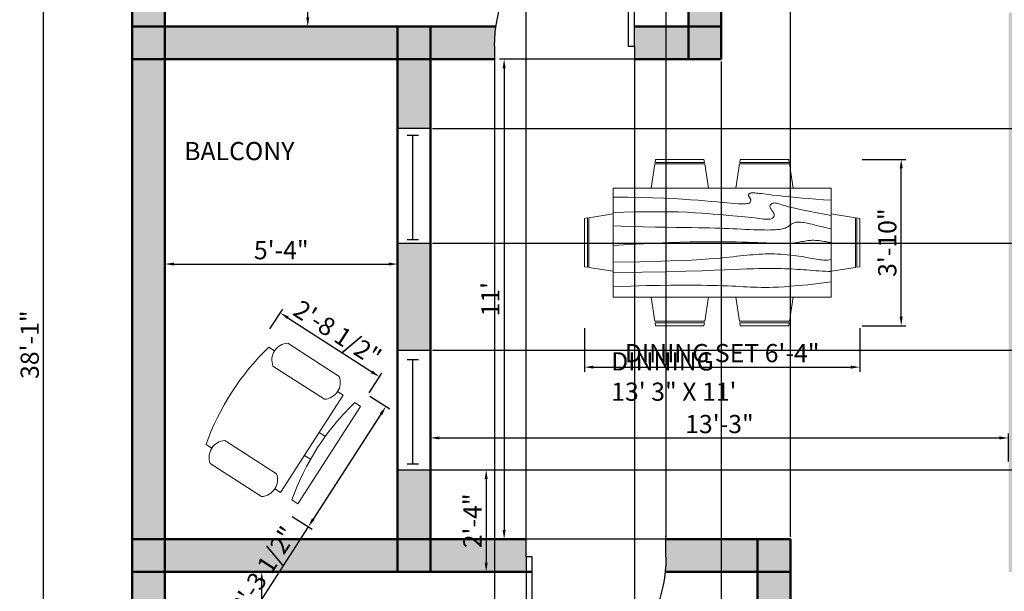
# Model space of a CAD drawing. Units: millimetres. Extents: x 3012 to 3478, y 929 to 1463.
# Tile 2 of 4: x 3012 to 3283, y 1118 to 1275. Entities that reach past the tile are written whole.
import ezdxf

# ---------------------------------------------------------------- set-up
doc = ezdxf.new("R2010")
doc.units = ezdxf.units.MM
for name, color, linetype, lineweight in [('A-ANNO-DIMS', 50, 'Continuous', 18), ('A-AREA-IDEN', 170, 'Continuous', 25), ('A-WALL-PATT', 252, 'Continuous', 13), ('doors', 130, 'Continuous', 25), ('furniture', 80, 'Continuous', 18), ('walls', 10, 'Continuous', 50), ('windows', 40, 'Continuous', 25)]:
    doc.layers.add(name, color=color, linetype=linetype, lineweight=lineweight)
doc.styles.get("Standard").update_dxf_attribs({"font": 'arial.ttf'})
doc.dimstyles.new('ISO-25', dxfattribs={"dimtxt": 5, "dimasz": 2.5, "dimexe": 1.25, "dimexo": 0.625, "dimtad": 1, "dimdec": 0, "dimlunit": 3, "dimtxsty": 'Standard', "dimcen": 2.5, "dimadec": 0, "dimazin": 0, "dimtfac": 1, "dimtdec": 0, "dimtmove": 0, "dimatfit": 3, "dimfxl": 1, "dimarcsym": 0})

# ---------------------------------------------------------------- blocks, each defined once
blk = doc.blocks.new('*U2')
for p, q in [((0, 0), (0, -6)), ((40, 0), (40, -6))]:
    blk.add_line(p, q)
blk.add_lwpolyline([(0, 0), (0, 40), (1.75, 40), (1.75, 0)], close=True)
blk.add_arc((0, 0), 40, 0, 90)
blk = doc.blocks.new('*U4')
for p, q in [((0, 4), (0, 0)), ((36, 4), (36, 0)), ((0, 2), (36, 2))]:
    blk.add_line(p, q)
blk = doc.blocks.new('Dining Set - 36 x 72 in.')
for p, q in [((-22, 27.5), (-22.1562, 26.50042)), ((-5.8416, 26.5), (-22.1534, 26.5)), ((-22, 27.5), (-6, 27.5)), ((-5.8437, 26.49966), (-6, 27.5)), ((6, 27.5), (5.8438, 26.50042)), ((22.1584, 26.5), (5.8466, 26.5)), ((6, 27.5), (22, 27.5)), ((22.1563, 26.49966), (22, 27.5)), ((-22.2343, 26.00059), (-23.4847, 17.99762)), ((-22.2304, 26), (-5.7608, 26)), ((-4.5152, 17.99762), (-5.7655, 25.99926)), ((5.7657, 26.00059), (4.5153, 17.99762)), ((5.7696, 26), (22.2392, 26)), ((23.4848, 17.99762), (22.2345, 25.99926)), ((36, 18), (-36, 18)), ((-36, 18), (-36, -18)), ((36, -18), (36, 18)), ((-45.5, 8), (-44.5004, 8.15617)), ((-45.5, 8), (-45.5, -8)), ((-44.5, -8.15843), (-44.5, 8.15338)), ((-44.0006, 8.23428), (-35.9976, 9.48474)), ((-44, 8.23041), (-44, -8.23915)), ((44.0006, 8.23428), (35.9976, 9.48474)), ((44, 8.23041), (44, -8.23915)), ((44.5, -8.15843), (44.5, 8.15338)), ((45.5, 8), (44.5005, 8.15617)), ((45.5, 8), (45.5, -8)), ((-44.4997, -8.15631), (-45.5, -8)), ((-35.9976, -9.48476), (-43.9993, -8.2345)), ((35.9976, -9.48476), (43.9993, -8.2345)), ((44.4997, -8.15631), (45.5, -8)), ((-36, -18), (36, -18)), ((-22.2343, -26.0006), (-23.4847, -17.99762)), ((-4.5152, -17.99762), (-5.7655, -25.99928)), ((5.7657, -26.0006), (4.5153, -17.99762)), ((23.4848, -17.99762), (22.2345, -25.99928)), ((-22.2304, -26), (-5.7608, -26)), ((5.7696, -26), (22.2392, -26)), ((-22, -27.5), (-22.1562, -26.50044)), ((-5.8416, -26.5), (-22.1534, -26.5)), ((-22, -27.5), (-6, -27.5)), ((-5.8437, -26.49967), (-6, -27.5)), ((6, -27.5), (5.8438, -26.50044)), ((22.1584, -26.5), (5.8466, -26.5)), ((6, -27.5), (22, -27.5)), ((22.1563, -26.49967), (22, -27.5))]:
    blk.add_line(p, q)
for points in [[(-36, 15), (-31.1772, 14.97754), (-26.8079, 14.91406), (-22.8538, 14.81543), (-19.276, 14.6875), (-16.0362, 14.53613), (-13.0957, 14.36718), (-10.4159, 14.18652), (-7.9583, 14), (-5.6904, 13.81315), (-3.6035, 13.63021), (-1.6954, 13.45508), (0.0365, 13.29166), (1.5945, 13.14388), (2.9811, 13.01562), (4.1988, 12.9108), (5.25, 12.83333), (6.1393, 12.78613), (6.8802, 12.76823), (7.4883, 12.77767), (7.9792, 12.8125), (8.3685, 12.87077), (8.6719, 12.95052), (8.9049, 13.0498), (9.0833, 13.16666), (9.2205, 13.29899), (9.3216, 13.44401), (9.3895, 13.59879), (9.4271, 13.76041), (9.4373, 13.92594), (9.4232, 14.09245), (9.3875, 14.257), (9.3333, 14.41666), (9.2638, 14.56917), (9.1836, 14.71484), (9.0975, 14.85465), (9.0104, 14.98958), (8.9272, 15.1206), (8.8529, 15.2487), (8.7922, 15.37483), (8.75, 15.5), (8.7305, 15.62467), (8.7344, 15.74739), (8.7617, 15.86621), (8.8125, 15.97916), (8.8867, 16.08431), (8.9844, 16.17968), (9.1055, 16.26334), (9.25, 16.33333), (9.4189, 16.38802), (9.6172, 16.42708), (9.8506, 16.45052), (10.125, 16.45833), (10.4463, 16.45052), (10.8203, 16.42708), (11.2529, 16.38802), (11.75, 16.33333), (12.3184, 16.26318), (12.9694, 16.17838), (13.7151, 16.07991), (14.5677, 15.96875), (15.5395, 15.84586), (16.6426, 15.71224), (17.8893, 15.56884), (19.2917, 15.41666), (20.859, 15.25667), (22.5879, 15.08984), (24.4721, 14.91715), (26.5052, 14.73958), (28.6809, 14.5581), (30.9929, 14.3737), (33.4347, 14.18733), (36, 14)], [(-36, 10), (-28.9766, 10.14274), (-23.1725, 10.20442), (-18.4241, 10.19775), (-14.5677, 10.13541), (-11.4399, 10.03011), (-8.877, 9.89453), (-6.7154, 9.74137), (-4.7917, 9.58333), (-2.9698, 9.43082), (-1.2246, 9.28515), (0.4415, 9.14534), (2.026, 9.01041), (3.5266, 8.87939), (4.9408, 8.7513), (6.266, 8.62516), (7.5, 8.5), (8.6411, 8.37549), (9.6914, 8.2539), (10.6538, 8.13818), (11.5312, 8.03125), (12.3267, 7.93603), (13.043, 7.85547), (13.6831, 7.79248), (14.25, 7.75), (14.7471, 7.7303), (15.1797, 7.73307), (15.5537, 7.75732), (15.875, 7.80208), (16.1494, 7.86637), (16.3828, 7.94922), (16.5811, 8.04964), (16.75, 8.16666), (16.8944, 8.29915), (17.0143, 8.44531), (17.1089, 8.60319), (17.1771, 8.77083), (17.218, 8.94629), (17.2305, 9.1276), (17.2137, 9.31282), (17.1667, 9.5), (17.0895, 9.6875), (16.987, 9.875), (16.8649, 10.0625), (16.7292, 10.25), (16.5856, 10.4375), (16.4401, 10.625), (16.2985, 10.8125), (16.1667, 11), (16.05, 11.18733), (15.9518, 11.3737), (15.8752, 11.5581), (15.8229, 11.73958), (15.798, 11.91715), (15.8034, 12.08984), (15.842, 12.25667), (15.9167, 12.41666), (16.0295, 12.56836), (16.1784, 12.70833), (16.3605, 12.83268), (16.5729, 12.9375), (16.8127, 13.01888), (17.0768, 13.07291), (17.3625, 13.0957), (17.6667, 13.08333), (17.9894, 13.03312), (18.3418, 12.94726), (18.7382, 12.82918), (19.1927, 12.68229), (19.7195, 12.51001), (20.3327, 12.31575), (21.0465, 12.10294), (21.875, 11.875), (22.8357, 11.63354), (23.959, 11.37304), (25.2786, 11.08618), (26.8282, 10.76562), (28.6414, 10.40405), (30.752, 9.99414), (33.1936, 9.52856), (36, 9)], [(-36, 5.5), (-30.7157, 5.3348), (-26.069, 5.20963), (-21.9946, 5.11767), (-18.4271, 5.05208), (-15.3009, 5.00602), (-12.5508, 4.97265), (-10.1112, 4.94515), (-7.9167, 4.91666), (-5.909, 4.88167), (-4.0586, 4.83984), (-2.3429, 4.79215), (-0.7396, 4.73958), (0.7739, 4.6831), (2.22, 4.6237), (3.6213, 4.56233), (5, 4.5), (6.373, 4.43782), (7.7344, 4.3776), (9.0723, 4.32129), (10.375, 4.27083), (11.6309, 4.22819), (12.8281, 4.19531), (13.9551, 4.17415), (15, 4.16666), (15.954, 4.17448), (16.819, 4.19791), (17.6001, 4.23698), (18.3021, 4.29166), (18.9299, 4.36198), (19.4883, 4.44791), (19.9823, 4.54948), (20.4167, 4.66666), (20.7969, 4.79899), (21.1302, 4.94401), (21.4245, 5.09879), (21.6875, 5.26041), (21.9271, 5.42594), (22.1511, 5.59245), (22.3672, 5.757), (22.5834, 5.91666), (22.8065, 6.06868), (23.0404, 6.21093), (23.2879, 6.34147), (23.5521, 6.45833), (23.8358, 6.55957), (24.142, 6.64323), (24.4735, 6.70735), (24.8334, 6.75), (25.2235, 6.76969), (25.642, 6.76692), (26.0858, 6.74267), (26.5521, 6.69791), (27.0379, 6.63362), (27.5404, 6.55078), (28.0565, 6.45036), (28.5834, 6.33333), (29.1242, 6.19987), (29.7071, 6.04687), (30.3661, 5.87044), (31.1354, 5.66666), (32.0493, 5.43164), (33.142, 5.16146), (34.4475, 4.85221), (36, 4.5)], [(-36, -1), (-30.7915, -0.6591), (-26.0195, -0.38216), (-21.6519, -0.16284), (-17.6563, 0.00521), (-14.0005, 0.12833), (-10.6523, 0.21289), (-7.5796, 0.26522), (-4.75, 0.29166), (-2.134, 0.29793), (0.2878, 0.28711), (2.5317, 0.26163), (4.6146, 0.22396), (6.5529, 0.17651), (8.3633, 0.12174), (10.0623, 0.06209), (11.6667, 0), (13.1899, -0.06201), (14.6341, -0.1211), (15.9982, -0.17432), (17.2813, -0.21875), (18.4823, -0.25147), (19.6003, -0.26953), (20.6343, -0.27002), (21.5834, -0.25), (22.4481, -0.20768), (23.2357, -0.14584), (23.9549, -0.06836), (24.6146, 0.02083), (25.2235, 0.11784), (25.7904, 0.21875), (26.3241, 0.31966), (26.8334, 0.41666), (27.3265, 0.50618), (27.8099, 0.58593), (28.2894, 0.65397), (28.7709, 0.70833), (29.2601, 0.74707), (29.763, 0.76823), (30.2855, 0.76985), (30.8334, 0.75), (31.4088, 0.70784), (31.9994, 0.64713), (32.589, 0.57275), (33.1615, 0.48958), (33.7008, 0.4025), (34.1908, 0.3164), (34.6153, 0.23616), (34.9584, 0.16666), (35.2099, 0.11165), (35.3848, 0.07031), (35.504, 0.04069), (35.5886, 0.02083), (35.6594, 0.00879), (35.7377, 0.0026), (35.8442, 0.00032), (36, 0)], [(-36, -6.5), (-27.1843, -6.31267), (-20.084, -6.1263), (-14.469, -5.9419), (-10.1094, -5.76042), (-6.7752, -5.58285), (-4.2363, -5.41016), (-2.2629, -5.24333), (-0.625, -5.08334), (0.8708, -4.93099), (2.2715, -4.78646), (3.5872, -4.64974), (4.8281, -4.52084), (6.0046, -4.39974), (7.127, -4.28646), (8.2053, -4.18099), (9.25, -4.08334), (10.2705, -3.99382), (11.2734, -3.91407), (12.2647, -3.84603), (13.25, -3.79167), (14.2354, -3.75293), (15.2266, -3.73177), (16.2295, -3.73015), (17.25, -3.75), (18.2912, -3.79248), (19.3451, -3.85547), (20.4009, -3.93604), (21.4479, -4.03125), (22.4754, -4.13819), (23.4727, -4.25391), (24.4289, -4.37549), (25.3334, -4.5), (26.1785, -4.62492), (26.9694, -4.74935), (27.7145, -4.87281), (28.4219, -4.99479), (29.1, -5.11483), (29.7572, -5.23242), (30.4016, -5.34709), (31.0417, -5.45834), (31.6837, -5.56437), (32.3262, -5.65821), (32.9658, -5.73153), (33.599, -5.77604), (34.2224, -5.78345), (34.8327, -5.74545), (35.4264, -5.65373), (36, -5.5)], [(-36, -10), (-26.4022, -9.81299), (-18.4675, -9.62891), (-11.9839, -9.45069), (-6.7396, -9.28125), (-2.5226, -9.12354), (0.8789, -8.98047), (3.6769, -8.85498), (6.0833, -8.75), (8.2767, -8.66765), (10.3021, -8.60677), (12.1712, -8.56543), (13.8958, -8.54167), (15.4876, -8.53353), (16.9583, -8.53907), (18.3197, -8.55632), (19.5834, -8.58334), (20.7616, -8.61841), (21.8685, -8.66081), (22.9188, -8.71004), (23.9271, -8.76563), (24.9081, -8.82707), (25.8763, -8.89388), (26.8465, -8.96558), (27.8334, -9.04167), (28.8474, -9.12118), (29.8828, -9.20117), (30.93, -9.27824), (31.9792, -9.34896), (33.0205, -9.40991), (34.0443, -9.45768), (35.0407, -9.48885), (36, -9.5)], [(-36, -14.5), (-30.0881, -14.33513), (-25.0332, -14.21224), (-20.7312, -14.12647), (-17.0781, -14.07292), (-13.97, -14.04671), (-11.3027, -14.04297), (-8.9724, -14.05681), (-6.875, -14.08334), (-4.9224, -14.11833), (-3.0905, -14.16016), (-1.3709, -14.20785), (0.2448, -14.26042), (1.7647, -14.3169), (3.1973, -14.3763), (4.5507, -14.43767), (5.8333, -14.5), (7.0554, -14.5621), (8.235, -14.62175), (9.3922, -14.67652), (10.5469, -14.72396), (11.7192, -14.76164), (12.929, -14.78711), (14.1965, -14.79794), (15.5417, -14.79167), (16.9933, -14.76424), (18.6152, -14.70508), (20.4804, -14.60197), (22.6615, -14.44271), (25.2312, -14.21509), (28.2624, -13.9069), (31.8277, -13.50594), (36, -13)]]:
    blk.add_lwpolyline(points)
blk = doc.blocks.new('Chair - Desk')
for p, q in [((-8.5, 0), (-8.5, -1)), ((-8.5, 0), (8.5, 0)), ((8.5, 0), (8.5, -1)), ((-2, -3), (-2, -1.9355)), ((2, -1.9576), (2, -3)), ((-8.5, -3), (-8.5, -4)), ((-8.5, -3), (8.5, -3)), ((8.5, -3), (8.5, -4)), ((-10.5, -5), (-10.5, -14)), ((-6.5, -14), (-6.5, -5)), ((6.5, -5), (6.5, -14)), ((10.5, -14), (10.5, -5)), ((-8.5, -15), (-8.5, -16)), ((8.5, -15), (8.5, -16))]:
    blk.add_line(p, q)
for centre, radius, start, end in [((0, 34.625), 36.625, 256.5803, 283.4197), ((-8.5, -6.5), 2.5, 36.8699, 143.1301), ((8.5, -6.5), 2.5, 36.8699, 143.1301), ((-8.5, -12.5), 2.5, 216.8699, 323.1301), ((8.5, -12.5), 2.5, 216.8699, 323.1301), ((0, 19.625), 36.625, 256.5803, 283.4197)]:
    blk.add_arc(centre, radius, start, end)
blk = doc.blocks.new('*D13')
at = {"layer": 'A-ANNO-DIMS', "color": 0, "lineweight": -2, "transparency": 16777216}
for p, q in [((3089.79, 1405.44), (3092.75, 1405.44)), ((3091.5, 1275.94), (3091.5, 1402.94)), ((3089.79, 1273.44), (3092.75, 1273.44))]:
    blk.add_line(p, q, dxfattribs=at)
at = {"layer": 'A-ANNO-DIMS', "color": 0, "transparency": 16777216}
for points in [[(3091.08, 1402.94), (3091.91, 1402.94), (3091.5, 1405.44)], [(3091.08, 1275.94), (3091.91, 1275.94), (3091.5, 1273.44)]]:
    blk.add_solid(points, dxfattribs=at)
at = {"layer": 'Defpoints', "color": 0, "transparency": 16777216}
for p in [(3089.17, 1405.44), (3091.5, 1405.44), (3089.17, 1273.44)]:
    blk.add_point(p, dxfattribs=at)
at = {"layer": 'A-ANNO-DIMS', "color": 0, "transparency": 16777216, "insert": (3088.36, 1339.44), "char_height": 5, "attachment_point": 5, "rotation": 90}
blk.add_mtext("11'", dxfattribs=at)
blk = doc.blocks.new('*D17')
at = {"layer": 'A-ANNO-DIMS', "color": 0, "lineweight": -2, "transparency": 16777216}
for p, q in [((3052.21, 1203.36), (3052.21, 1209.37)), ((3054.71, 1208.12), (3113.71, 1208.12)), ((3116.21, 1203.36), (3116.21, 1209.37))]:
    blk.add_line(p, q, dxfattribs=at)
at = {"layer": 'A-ANNO-DIMS', "color": 0, "transparency": 16777216}
for points in [[(3054.71, 1208.53), (3054.71, 1207.7), (3052.21, 1208.12)], [(3113.71, 1208.53), (3113.71, 1207.7), (3116.21, 1208.12)]]:
    blk.add_solid(points, dxfattribs=at)
at = {"layer": 'Defpoints', "color": 0, "transparency": 16777216}
for p in [(3116.21, 1208.12), (3052.21, 1202.73), (3116.21, 1202.73)]:
    blk.add_point(p, dxfattribs=at)
at = {"layer": 'A-ANNO-DIMS', "color": 0, "transparency": 16777216, "insert": (3084.21, 1211.28), "char_height": 5, "attachment_point": 5}
blk.add_mtext('5\'-4"', dxfattribs=at)
blk = doc.blocks.new('*D19')
at = {"layer": 'A-ANNO-DIMS', "color": 0, "lineweight": -2, "transparency": 16777216}
for p, q in [((3065.42, 1123.44), (3080.09, 1123.44)), ((3078.84, 968.94), (3078.84, 1120.94)), ((3065.42, 966.44), (3080.09, 966.44))]:
    blk.add_line(p, q, dxfattribs=at)
at = {"layer": 'A-ANNO-DIMS', "color": 0, "transparency": 16777216}
for points in [[(3078.43, 1120.94), (3079.26, 1120.94), (3078.84, 1123.44)], [(3078.43, 968.94), (3079.26, 968.94), (3078.84, 966.44)]]:
    blk.add_solid(points, dxfattribs=at)
at = {"layer": 'Defpoints', "color": 0, "transparency": 16777216}
for p in [(3064.8, 1123.44), (3078.84, 1123.44), (3064.8, 966.44)]:
    blk.add_point(p, dxfattribs=at)
at = {"layer": 'A-ANNO-DIMS', "color": 0, "transparency": 16777216, "insert": (3075.66, 1044.94), "char_height": 5, "attachment_point": 5, "rotation": 90}
blk.add_mtext('13\'-1"', dxfattribs=at)
blk = doc.blocks.new('*D25')
at = {"layer": 'A-ANNO-DIMS', "color": 0, "lineweight": -2, "transparency": 16777216}
for p, q in [((3125.21, 1153.8), (3125.21, 1161.53)), ((3127.71, 1160.28), (3281.71, 1160.28)), ((3284.21, 1153.8), (3284.21, 1161.53))]:
    blk.add_line(p, q, dxfattribs=at)
at = {"layer": 'A-ANNO-DIMS', "color": 0, "transparency": 16777216}
for points in [[(3127.71, 1160.7), (3127.71, 1159.86), (3125.21, 1160.28)], [(3281.71, 1160.7), (3281.71, 1159.86), (3284.21, 1160.28)]]:
    blk.add_solid(points, dxfattribs=at)
at = {"layer": 'Defpoints', "color": 0, "transparency": 16777216}
for p in [(3284.21, 1160.28), (3125.21, 1153.17), (3284.21, 1153.17)]:
    blk.add_point(p, dxfattribs=at)
at = {"layer": 'A-ANNO-DIMS', "color": 0, "transparency": 16777216, "insert": (3204.71, 1163.46), "char_height": 5, "attachment_point": 5}
blk.add_mtext('13\'-3"', dxfattribs=at)
blk = doc.blocks.new('*D26')
at = {"layer": 'A-ANNO-DIMS', "color": 0, "lineweight": -2, "transparency": 16777216}
for p, q in [((3195.59, 1264.44), (3144.25, 1264.44)), ((3145.5, 1261.94), (3145.5, 1134.94)), ((3195.59, 1132.44), (3144.25, 1132.44))]:
    blk.add_line(p, q, dxfattribs=at)
at = {"layer": 'A-ANNO-DIMS', "color": 0, "transparency": 16777216}
for points in [[(3145.08, 1261.94), (3145.92, 1261.94), (3145.5, 1264.44)], [(3145.08, 1134.94), (3145.92, 1134.94), (3145.5, 1132.44)]]:
    blk.add_solid(points, dxfattribs=at)
at = {"layer": 'Defpoints', "color": 0, "transparency": 16777216}
for p in [(3196.21, 1264.44), (3145.5, 1132.44), (3196.21, 1132.44)]:
    blk.add_point(p, dxfattribs=at)
at = {"layer": 'A-ANNO-DIMS', "color": 0, "transparency": 16777216, "insert": (3142.36, 1198.44), "char_height": 5, "attachment_point": 5, "rotation": 90}
blk.add_mtext("11'", dxfattribs=at)
blk = doc.blocks.new('*D34')
at = {"layer": 'A-ANNO-DIMS', "color": 0, "lineweight": -2, "transparency": 16777216}
for p, q in [((3167.57, 1190.5), (3167.57, 1178.51)), ((3243.33, 1190.5), (3243.33, 1178.51)), ((3170.07, 1179.76), (3240.83, 1179.76))]:
    blk.add_line(p, q, dxfattribs=at)
at = {"layer": 'A-ANNO-DIMS', "color": 0, "transparency": 16777216}
for points in [[(3170.07, 1180.17), (3170.07, 1179.34), (3167.57, 1179.76)], [(3240.83, 1180.17), (3240.83, 1179.34), (3243.33, 1179.76)]]:
    blk.add_solid(points, dxfattribs=at)
at = {"layer": 'Defpoints', "color": 0, "transparency": 16777216}
for p in [(3167.57, 1191.12), (3243.33, 1191.12), (3243.33, 1179.76)]:
    blk.add_point(p, dxfattribs=at)
at = {"layer": 'A-ANNO-DIMS', "color": 0, "transparency": 16777216, "insert": (3205.45, 1182.97), "char_height": 5, "attachment_point": 5}
blk.add_mtext('DINING SET 6\'-4"', dxfattribs=at)
blk = doc.blocks.new('*D35')
at = {"layer": 'A-ANNO-DIMS', "color": 0, "lineweight": -2, "transparency": 16777216}
for p, q in [((3243.95, 1236.91), (3255.94, 1236.91)), ((3254.69, 1193.62), (3254.69, 1234.41)), ((3243.95, 1191.12), (3255.94, 1191.12))]:
    blk.add_line(p, q, dxfattribs=at)
at = {"layer": 'A-ANNO-DIMS', "color": 0, "transparency": 16777216}
for points in [[(3254.27, 1234.41), (3255.11, 1234.41), (3254.69, 1236.91)], [(3254.27, 1193.62), (3255.11, 1193.62), (3254.69, 1191.12)]]:
    blk.add_solid(points, dxfattribs=at)
at = {"layer": 'Defpoints', "color": 0, "transparency": 16777216}
for p in [(3243.33, 1236.91), (3254.69, 1236.91), (3243.33, 1191.12)]:
    blk.add_point(p, dxfattribs=at)
at = {"layer": 'A-ANNO-DIMS', "color": 0, "transparency": 16777216, "insert": (3251.51, 1214.01), "char_height": 5, "attachment_point": 5, "rotation": 90}
blk.add_mtext('3\'-10"', dxfattribs=at)
blk = doc.blocks.new('*D40')
at = {"layer": 'A-ANNO-DIMS', "color": 0, "lineweight": -2, "transparency": 16777216}
for p, q in [((3108.55, 1171.79), (3114.04, 1168.25)), ((3111.63, 1166.83), (3093, 1137.95)), ((3087.21, 1138.72), (3092.7, 1135.18)), ((3091.65, 1135.85), (3063.29, 1091.9))]:
    blk.add_line(p, q, dxfattribs=at)
at = {"layer": 'A-ANNO-DIMS', "color": 0, "transparency": 16777216}
for points in [[(3111.28, 1167.05), (3111.98, 1166.6), (3112.99, 1168.93)], [(3092.65, 1138.18), (3093.35, 1137.73), (3091.65, 1135.85)]]:
    blk.add_solid(points, dxfattribs=at)
at = {"layer": 'Defpoints', "color": 0, "transparency": 16777216}
for p in [(3108.03, 1172.13), (3086.69, 1139.06), (3091.65, 1135.85)]:
    blk.add_point(p, dxfattribs=at)
at = {"layer": 'A-ANNO-DIMS', "color": 0, "transparency": 16777216, "insert": (3074.09, 1114.57), "char_height": 5, "attachment_point": 5, "rotation": 57.1659}
blk.add_mtext('CHAIR 3\'-3 1/2"', dxfattribs=at)
blk = doc.blocks.new('*D41')
at = {"layer": 'A-ANNO-DIMS', "color": 0, "lineweight": -2, "transparency": 16777216}
for p, q in [((3081.07, 1190.27), (3084.61, 1195.75)), ((3086.03, 1193.35), (3109.13, 1178.44)), ((3108.37, 1172.65), (3111.91, 1178.14))]:
    blk.add_line(p, q, dxfattribs=at)
at = {"layer": 'A-ANNO-DIMS', "color": 0, "transparency": 16777216}
for points in [[(3086.26, 1193.7), (3085.81, 1193), (3083.93, 1194.7)], [(3109.35, 1178.79), (3108.9, 1178.09), (3111.23, 1177.09)]]:
    blk.add_solid(points, dxfattribs=at)
at = {"layer": 'Defpoints', "color": 0, "transparency": 16777216}
for p in [(3080.73, 1189.74), (3111.23, 1177.09), (3108.03, 1172.13)]:
    blk.add_point(p, dxfattribs=at)
at = {"layer": 'A-ANNO-DIMS', "color": 0, "transparency": 16777216, "insert": (3099.32, 1188.59), "char_height": 5, "attachment_point": 5, "rotation": 327.1659}
blk.add_mtext('2\'-8 1/2"', dxfattribs=at)
blk = doc.blocks.new('*D42')
at = {"layer": 'A-ANNO-DIMS', "color": 0, "lineweight": -2, "transparency": 16777216}
for p, q in [((3042.59, 1414.44), (3017.61, 1414.44)), ((3018.86, 959.94), (3018.86, 1411.94)), ((3042.59, 957.44), (3017.61, 957.44))]:
    blk.add_line(p, q, dxfattribs=at)
at = {"layer": 'A-ANNO-DIMS', "color": 0, "transparency": 16777216}
for points in [[(3018.45, 1411.94), (3019.28, 1411.94), (3018.86, 1414.44)], [(3018.45, 959.94), (3019.28, 959.94), (3018.86, 957.44)]]:
    blk.add_solid(points, dxfattribs=at)
at = {"layer": 'Defpoints', "color": 0, "transparency": 16777216}
for p in [(3018.86, 1414.44), (3043.21, 1414.44), (3043.21, 957.44)]:
    blk.add_point(p, dxfattribs=at)
at = {"layer": 'A-ANNO-DIMS', "color": 0, "transparency": 16777216, "insert": (3015.68, 1185.94), "char_height": 5, "attachment_point": 5, "rotation": 90}
blk.add_mtext('38\'-1"', dxfattribs=at)
blk = doc.blocks.new('*D57')
at = {"layer": 'A-ANNO-DIMS', "color": 0, "lineweight": -2, "transparency": 16777216}
for p, q in [((3142.87, 1263.82), (3142.87, 931.84)), ((3181.32, 1263.82), (3181.32, 931.84)), ((3145.37, 933.09), (3178.82, 933.09))]:
    blk.add_line(p, q, dxfattribs=at)
at = {"layer": 'A-ANNO-DIMS', "color": 0, "transparency": 16777216}
for points in [[(3145.37, 933.51), (3145.37, 932.68), (3142.87, 933.09)], [(3178.82, 933.51), (3178.82, 932.68), (3181.32, 933.09)]]:
    blk.add_solid(points, dxfattribs=at)
at = {"layer": 'Defpoints', "color": 0, "transparency": 16777216}
for p in [(3142.87, 1264.44), (3181.32, 1264.44), (3181.32, 933.09)]:
    blk.add_point(p, dxfattribs=at)
at = {"layer": 'A-ANNO-DIMS', "color": 0, "transparency": 16777216, "insert": (3162.1, 936.3), "char_height": 5, "attachment_point": 5}
blk.add_mtext('3\'-2 1/2"', dxfattribs=at)
blk = doc.blocks.new('*D58')
at = {"layer": 'A-ANNO-DIMS', "color": 0, "lineweight": -2, "transparency": 16777216}
for p, q in [((3181.32, 1263.82), (3181.32, 931.84)), ((3205.21, 1263.82), (3205.21, 931.84)), ((3183.82, 933.09), (3202.71, 933.09))]:
    blk.add_line(p, q, dxfattribs=at)
at = {"layer": 'A-ANNO-DIMS', "color": 0, "transparency": 16777216}
for points in [[(3183.82, 933.51), (3183.82, 932.68), (3181.32, 933.09)], [(3202.71, 933.51), (3202.71, 932.68), (3205.21, 933.09)]]:
    blk.add_solid(points, dxfattribs=at)
at = {"layer": 'Defpoints', "color": 0, "transparency": 16777216}
for p in [(3181.32, 1264.44), (3205.21, 1264.44), (3205.21, 933.09)]:
    blk.add_point(p, dxfattribs=at)
at = {"layer": 'A-ANNO-DIMS', "color": 0, "transparency": 16777216, "insert": (3193.27, 936.27), "char_height": 5, "attachment_point": 5}
blk.add_mtext('2\'-0"', dxfattribs=at)
blk = doc.blocks.new('*D61')
at = {"layer": 'A-ANNO-DIMS', "color": 0, "lineweight": -2, "transparency": 16777216}
for p, q in [((3151.56, 1133.07), (3151.56, 1440.04)), ((3154.06, 1438.79), (3187.51, 1438.79)), ((3190.01, 1133.07), (3190.01, 1440.04))]:
    blk.add_line(p, q, dxfattribs=at)
at = {"layer": 'A-ANNO-DIMS', "color": 0, "transparency": 16777216}
for points in [[(3154.06, 1439.21), (3154.06, 1438.38), (3151.56, 1438.79)], [(3187.51, 1439.21), (3187.51, 1438.38), (3190.01, 1438.79)]]:
    blk.add_solid(points, dxfattribs=at)
at = {"layer": 'Defpoints', "color": 0, "transparency": 16777216}
for p in [(3190.01, 1438.79), (3151.56, 1132.44), (3190.01, 1132.44)]:
    blk.add_point(p, dxfattribs=at)
at = {"layer": 'A-ANNO-DIMS', "color": 0, "transparency": 16777216, "insert": (3170.79, 1442), "char_height": 5, "attachment_point": 5}
blk.add_mtext('3\'-2 1/2"', dxfattribs=at)
blk = doc.blocks.new('*D62')
at = {"layer": 'A-ANNO-DIMS', "color": 0, "lineweight": -2, "transparency": 16777216}
for p, q in [((3190.01, 1133.07), (3190.01, 1440.04)), ((3192.51, 1438.79), (3221.71, 1438.79)), ((3224.21, 1133.07), (3224.21, 1440.04))]:
    blk.add_line(p, q, dxfattribs=at)
at = {"layer": 'A-ANNO-DIMS', "color": 0, "transparency": 16777216}
for points in [[(3192.51, 1439.21), (3192.51, 1438.38), (3190.01, 1438.79)], [(3221.71, 1439.21), (3221.71, 1438.38), (3224.21, 1438.79)]]:
    blk.add_solid(points, dxfattribs=at)
at = {"layer": 'Defpoints', "color": 0, "transparency": 16777216}
for p in [(3224.21, 1438.79), (3190.01, 1132.44), (3224.21, 1132.44)]:
    blk.add_point(p, dxfattribs=at)
at = {"layer": 'A-ANNO-DIMS', "color": 0, "transparency": 16777216, "insert": (3207.11, 1441.97), "char_height": 5, "attachment_point": 5}
blk.add_mtext('2\'-10"', dxfattribs=at)
blk = doc.blocks.new('*D67')
at = {"layer": 'A-ANNO-DIMS', "color": 0, "lineweight": -2, "transparency": 16777216}
for p, q in [((3116.84, 1151.51), (3141.81, 1151.51)), ((3140.56, 1149.01), (3140.56, 1125.94)), ((3116.84, 1123.44), (3141.81, 1123.44))]:
    blk.add_line(p, q, dxfattribs=at)
at = {"layer": 'A-ANNO-DIMS', "color": 0, "transparency": 16777216}
for points in [[(3140.15, 1149.01), (3140.98, 1149.01), (3140.56, 1151.51)], [(3140.15, 1125.94), (3140.98, 1125.94), (3140.56, 1123.44)]]:
    blk.add_solid(points, dxfattribs=at)
at = {"layer": 'Defpoints', "color": 0, "transparency": 16777216}
for p in [(3116.21, 1151.51), (3116.21, 1123.44), (3140.56, 1123.44)]:
    blk.add_point(p, dxfattribs=at)
at = {"layer": 'A-ANNO-DIMS', "color": 0, "transparency": 16777216, "insert": (3137.43, 1137.48), "char_height": 5, "attachment_point": 5, "rotation": 90}
blk.add_mtext('2\'-4"', dxfattribs=at)
blk = doc.blocks.new('*D68')
at = {"layer": 'A-ANNO-DIMS', "color": 0, "lineweight": -2, "transparency": 16777216}
for p, q in [((3125.84, 1245.36), (3475.4, 1245.36)), ((3474.15, 1216.36), (3474.15, 1242.86)), ((3125.84, 1213.86), (3475.4, 1213.86))]:
    blk.add_line(p, q, dxfattribs=at)
at = {"layer": 'A-ANNO-DIMS', "color": 0, "transparency": 16777216}
for points in [[(3473.74, 1242.86), (3474.57, 1242.86), (3474.15, 1245.36)], [(3473.74, 1216.36), (3474.57, 1216.36), (3474.15, 1213.86)]]:
    blk.add_solid(points, dxfattribs=at)
at = {"layer": 'Defpoints', "color": 0, "transparency": 16777216}
for p in [(3125.21, 1245.36), (3474.15, 1245.36), (3125.21, 1213.86)]:
    blk.add_point(p, dxfattribs=at)
at = {"layer": 'A-ANNO-DIMS', "color": 0, "transparency": 16777216, "insert": (3470.94, 1229.61), "char_height": 5, "attachment_point": 5, "rotation": 90}
blk.add_mtext('2\'-7 1/2"', dxfattribs=at)
blk = doc.blocks.new('*D69')
at = {"layer": 'A-ANNO-DIMS', "color": 0, "lineweight": -2, "transparency": 16777216}
for p, q in [((3125.84, 1213.86), (3475.4, 1213.86)), ((3474.15, 1186.92), (3474.15, 1211.36)), ((3125.84, 1184.42), (3475.4, 1184.42))]:
    blk.add_line(p, q, dxfattribs=at)
at = {"layer": 'A-ANNO-DIMS', "color": 0, "transparency": 16777216}
for points in [[(3473.74, 1211.36), (3474.57, 1211.36), (3474.15, 1213.86)], [(3473.74, 1186.92), (3474.57, 1186.92), (3474.15, 1184.42)]]:
    blk.add_solid(points, dxfattribs=at)
at = {"layer": 'Defpoints', "color": 0, "transparency": 16777216}
for p in [(3125.21, 1213.86), (3474.15, 1213.86), (3125.21, 1184.42)]:
    blk.add_point(p, dxfattribs=at)
at = {"layer": 'A-ANNO-DIMS', "color": 0, "transparency": 16777216, "insert": (3470.94, 1199.14), "char_height": 5, "attachment_point": 5, "rotation": 90}
blk.add_mtext('2\'-5 1/2"', dxfattribs=at)
blk = doc.blocks.new('*D70')
at = {"layer": 'A-ANNO-DIMS', "color": 0, "lineweight": -2, "transparency": 16777216}
for p, q in [((3125.84, 1184.42), (3475.4, 1184.42)), ((3474.15, 1154.01), (3474.15, 1181.92)), ((3125.84, 1151.51), (3475.4, 1151.51))]:
    blk.add_line(p, q, dxfattribs=at)
at = {"layer": 'A-ANNO-DIMS', "color": 0, "transparency": 16777216}
for points in [[(3473.74, 1181.92), (3474.57, 1181.92), (3474.15, 1184.42)], [(3473.74, 1154.01), (3474.57, 1154.01), (3474.15, 1151.51)]]:
    blk.add_solid(points, dxfattribs=at)
at = {"layer": 'Defpoints', "color": 0, "transparency": 16777216}
for p in [(3125.21, 1184.42), (3474.15, 1184.42), (3125.21, 1151.51)]:
    blk.add_point(p, dxfattribs=at)
at = {"layer": 'A-ANNO-DIMS', "color": 0, "transparency": 16777216, "insert": (3470.98, 1167.97), "char_height": 5, "attachment_point": 5, "rotation": 90}
blk.add_mtext('2\'-9"', dxfattribs=at)

msp = doc.modelspace()

# ---------------------------------------------------------------- hatches: boundary and pattern name
at = {"layer": 'A-WALL-PATT'}
h = msp.add_hatch(color=256, dxfattribs=at)
h.dxf.hatch_style = 1
h.paths.add_polyline_path([(3052.21, 1405.44), (3043.21, 1405.44), (3043.21, 1273.44), (3052.21, 1273.44)])
h.paths.add_polyline_path([(3052.21, 1273.44), (3043.21, 1273.44), (3043.21, 1264.44), (3052.21, 1264.44)])
h.paths.add_polyline_path([(3052.21, 1264.44), (3043.21, 1264.44), (3043.21, 1132.44), (3052.21, 1132.44)])
h.paths.add_polyline_path([(3116.21, 1273.44), (3052.21, 1273.44), (3052.21, 1264.44), (3116.21, 1264.44)])
h.paths.add_polyline_path([(3125.21, 1273.44), (3116.21, 1273.44), (3116.21, 1264.44), (3125.21, 1264.44)])
h.paths.add_polyline_path([(3143.26, 1273.44), (3125.21, 1273.44), (3125.21, 1264.44), (3142.87, 1264.44), (3142.87, 1268, -0.035543)])
h.paths.add_polyline_path([(3052.21, 1414.44), (3043.21, 1414.44), (3043.21, 1405.44), (3052.21, 1405.44)])
h.paths.add_polyline_path([(3096.89, 1414.44), (3052.21, 1414.44), (3052.21, 1405.44), (3096.89, 1405.44)])
h.paths.add_polyline_path([(3196.21, 1414.44), (3129.12, 1414.44), (3129.12, 1405.44), (3196.21, 1405.44)])
h.paths.add_polyline_path([(3205.21, 1414.44), (3196.21, 1414.44), (3196.21, 1405.44), (3205.21, 1405.44)])
h.paths.add_polyline_path([(3205.21, 1405.44), (3196.21, 1405.44), (3196.21, 1321.44), (3205.21, 1321.44)])
h.paths.add_polyline_path([(3205.21, 1321.44), (3196.21, 1321.44), (3196.21, 1312.44), (3205.21, 1312.44)])
h.paths.add_polyline_path([(3205.21, 1312.44), (3196.21, 1312.44), (3196.21, 1273.44), (3205.21, 1273.44)])
h.paths.add_polyline_path([(3284.21, 1321.44), (3205.21, 1321.44), (3205.21, 1312.44), (3284.21, 1312.44)])
h.paths.add_polyline_path([(3205.21, 1273.44), (3196.21, 1273.44), (3196.21, 1264.44), (3205.21, 1264.44)])
h.paths.add_polyline_path([(3196.21, 1273.44), (3181.32, 1273.44), (3181.32, 1268), (3181.32, 1264.44), (3196.21, 1264.44)])
h.paths.add_polyline_path([(3293.21, 1405.44), (3284.21, 1405.44), (3284.21, 1321.44), (3293.21, 1321.44)])
h.paths.add_polyline_path([(3293.21, 1414.44), (3284.21, 1414.44), (3284.21, 1405.44), (3293.21, 1405.44)])
h.paths.add_polyline_path([(3284.21, 1414.44), (3249.55, 1414.44), (3249.55, 1405.44), (3284.21, 1405.44)])
h.paths.add_polyline_path([(3221.79, 1414.44), (3205.21, 1414.44), (3205.21, 1405.44), (3221.79, 1405.44)])
h.paths.add_polyline_path([(3339.87, 1414.44), (3293.21, 1414.44), (3293.21, 1405.44), (3339.87, 1405.44)])
h.paths.add_polyline_path([(3437.21, 1414.44), (3373.17, 1414.44), (3373.17, 1405.44), (3437.21, 1405.44)])
h.paths.add_polyline_path([(3446.21, 1414.44), (3437.21, 1414.44), (3437.21, 1405.44), (3446.21, 1405.44)])
h.paths.add_polyline_path([(3446.21, 1405.44), (3437.21, 1405.44), (3437.21, 1273.44), (3446.21, 1273.44)])
h.paths.add_polyline_path([(3437.21, 1273.44), (3293.21, 1273.44), (3293.21, 1264.44), (3437.21, 1264.44)])
h.paths.add_polyline_path([(3446.21, 1273.44), (3437.21, 1273.44), (3437.21, 1264.44), (3446.21, 1264.44)])
h.paths.add_polyline_path([(3446.21, 1264.44), (3437.21, 1264.44), (3437.21, 1249.83), (3445.52, 1249.83), (3446.21, 1249.83)])
h.paths.add_polyline_path([(3293.21, 1264.44), (3284.21, 1264.44), (3284.21, 1132.44), (3293.21, 1132.44)])
h.paths.add_polyline_path([(3293.21, 1273.44), (3284.21, 1273.44), (3284.21, 1264.44), (3293.21, 1264.44)])
h.paths.add_polyline_path([(3293.21, 1277.22), (3287.47, 1277.22), (3284.21, 1277.22), (3284.21, 1273.44), (3293.21, 1273.44)])
h.paths.add_polyline_path([(3125.21, 1213.86), (3116.21, 1213.86), (3116.21, 1184.42), (3125.21, 1184.42)])
h.paths.add_polyline_path([(3125.21, 1264.44), (3116.21, 1264.44), (3116.21, 1245.36), (3125.21, 1245.36)])
h.paths.add_polyline_path([(3125.21, 1151.51), (3116.21, 1151.51), (3116.21, 1132.44), (3125.21, 1132.44)])
h.paths.add_polyline_path([(3125.21, 1132.44), (3116.21, 1132.44), (3116.21, 1123.44), (3125.21, 1123.44)])
h.paths.add_polyline_path([(3151.56, 1127.56), (3151.56, 1132.44), (3125.21, 1132.44), (3125.21, 1123.44), (3151.56, 1123.44)])
h.paths.add_polyline_path([(3116.21, 1132.44), (3052.21, 1132.44), (3052.21, 1123.44), (3116.21, 1123.44)])
h.paths.add_polyline_path([(3052.21, 1132.44), (3043.21, 1132.44), (3043.21, 1123.44), (3052.21, 1123.44)])
h.paths.add_polyline_path([(3052.21, 1123.44), (3043.21, 1123.44), (3043.21, 966.44), (3052.21, 966.44)])
h.paths.add_polyline_path([(3097.57, 966.44), (3052.21, 966.44), (3052.21, 957.44), (3097.57, 957.44)])
h.paths.add_polyline_path([(3052.21, 966.44), (3043.21, 966.44), (3043.21, 957.44), (3052.21, 957.44)])
h.paths.add_polyline_path([(3215.21, 966.44), (3131.05, 966.44), (3131.05, 957.44), (3215.21, 957.44)])
h.paths.add_polyline_path([(3224.21, 966.44), (3215.21, 966.44), (3215.21, 957.44), (3224.21, 957.44)])
h.paths.add_polyline_path([(3224.21, 1004.97, -0.051409), (3218.39, 1004.37), (3215.21, 1004.37), (3215.21, 966.44), (3224.21, 966.44)])
h.paths.add_polyline_path([(3239.46, 966.44), (3224.21, 966.44), (3224.21, 957.44), (3239.46, 957.44)])
h.paths.add_polyline_path([(3344.91, 966.44), (3266.71, 966.44), (3266.71, 957.44), (3344.91, 957.44)])
h.paths.add_polyline_path([(3293.21, 1018.44), (3284.21, 1018.44), (3284.21, 966.44), (3293.21, 966.44)])
h.paths.add_polyline_path([(3293.21, 1027.44), (3284.21, 1027.44), (3284.21, 1018.44), (3293.21, 1018.44)])
h.paths.add_polyline_path([(3293.21, 1074.44), (3284.21, 1074.44), (3284.21, 1027.44), (3293.21, 1027.44)])
h.paths.add_polyline_path([(3224.21, 1074.44), (3215.21, 1074.44), (3215.21, 1032.91), (3218.39, 1032.91), (3224.21, 1032.91)])
h.paths.add_polyline_path([(3224.21, 1123.44), (3215.21, 1123.44), (3215.21, 1083.44), (3224.21, 1083.44)])
h.paths.add_polyline_path([(3224.21, 1083.44), (3215.21, 1083.44), (3215.21, 1074.44), (3224.21, 1074.44)])
h.paths.add_polyline_path([(3284.21, 1083.44), (3224.21, 1083.44), (3224.21, 1074.44), (3284.21, 1074.44)])
h.paths.add_polyline_path([(3293.21, 1083.44), (3284.21, 1083.44), (3284.21, 1074.44), (3293.21, 1074.44)])
h.paths.add_polyline_path([(3215.21, 1132.44), (3190.01, 1132.44), (3190.01, 1127.56, -0.026825), (3189.79, 1123.44), (3215.21, 1123.44)])
h.paths.add_polyline_path([(3224.21, 1132.44), (3215.21, 1132.44), (3215.21, 1123.44), (3224.21, 1123.44)])
h.paths.add_polyline_path([(3437.21, 1132.44), (3293.21, 1132.44), (3293.21, 1123.44), (3437.21, 1123.44)])
h.paths.add_polyline_path([(3293.21, 1132.44), (3284.21, 1132.44), (3284.21, 1123.44), (3293.21, 1123.44)])
h.paths.add_polyline_path([(3446.21, 1132.44), (3437.21, 1132.44), (3437.21, 1123.44), (3446.21, 1123.44)])
h.paths.add_polyline_path([(3446.21, 1123.44), (3437.21, 1123.44), (3437.21, 1027.44), (3446.21, 1027.44)])
h.paths.add_polyline_path([(3446.21, 1221.29), (3445.52, 1221.29, -0.074007), (3437.21, 1222.53), (3437.21, 1132.44), (3446.21, 1132.44)])
h.paths.add_polyline_path([(3446.21, 1018.44), (3437.21, 1018.44), (3437.21, 966.44), (3446.21, 966.44)])
h.paths.add_polyline_path([(3446.21, 1027.44), (3437.21, 1027.44), (3437.21, 1018.44), (3446.21, 1018.44)])
h.paths.add_polyline_path([(3437.21, 1027.44), (3389.3, 1027.44), (3389.3, 1025.95), (3389.3, 1018.44), (3437.21, 1018.44)])
h.paths.add_polyline_path([(3360.77, 1025.95), (3360.77, 1027.44), (3293.21, 1027.44), (3293.21, 1018.44), (3361.77, 1018.44, -0.066618)])
h.paths.add_polyline_path([(3437.21, 966.44), (3375.49, 966.44), (3375.49, 957.44), (3437.21, 957.44)])
h.paths.add_polyline_path([(3446.21, 966.44), (3437.21, 966.44), (3437.21, 957.44), (3446.21, 957.44)])

# ---------------------------------------------------------------- linework, layer by layer
at = {"layer": 'walls'}
for p, q in [((3043.21, 1414.44), (3043.21, 957.44)), ((3052.21, 1414.44), (3052.21, 957.44)), ((3196.21, 1414.44), (3196.21, 1264.44)), ((3205.21, 1414.44), (3205.21, 1264.44)), ((3043.21, 1273.44), (3143.26, 1273.44)), ((3043.21, 1273.44), (3143.26, 1273.44)), ((3116.21, 1273.44), (3116.21, 1123.44)), ((3125.21, 1273.44), (3125.21, 1123.44)), ((3181.32, 1273.44), (3205.21, 1273.44)), ((3181.32, 1273.44), (3205.21, 1273.44)), ((3043.21, 1264.44), (3142.87, 1264.44)), ((3043.21, 1264.44), (3142.87, 1264.44)), ((3181.32, 1264.44), (3205.21, 1264.44)), ((3181.32, 1264.44), (3205.21, 1264.44)), ((3043.21, 1132.44), (3151.56, 1132.44)), ((3190.01, 1132.44), (3224.21, 1132.44)), ((3215.21, 1132.44), (3215.21, 1032.91)), ((3224.21, 1132.44), (3224.21, 1032.91)), ((3043.21, 1123.44), (3153.24, 1123.44)), ((3189.79, 1123.44), (3224.21, 1123.44))]:
    msp.add_line(p, q, dxfattribs=at)
at = {"layer": 'windows'}
for p, q in [((3125.21, 1245.36), (3116.21, 1245.36)), ((3116.21, 1213.86), (3125.21, 1213.86)), ((3116.21, 1184.42), (3125.21, 1184.42)), ((3116.21, 1151.51), (3125.21, 1151.51)), ((3125.21, 1151.51), (3125.21, 1151.51))]:
    msp.add_line(p, q, dxfattribs=at)

# ---------------------------------------------------------------- block references
at = {"layer": 'doors', "xscale": -0.9611587719732299, "yscale": 0.9611587719732299, "zscale": 0.9611587719732299}
msp.add_blockref('*U2', (3181.32, 1268), dxfattribs=at)
at = {"layer": 'doors', "xscale": -0.9611587719732299, "yscale": 0.9611587719732299, "zscale": 0.9611587719732299, "rotation": 180}
msp.add_blockref('*U2', (3151.56, 1127.56), dxfattribs=at)
at = {"layer": 'furniture', "xscale": 0.8325018186934077, "yscale": 0.8325018186934077, "zscale": 0.8325018186934077}
msp.add_blockref('Dining Set - 36 x 72 in.', (3205.45, 1214.01), dxfattribs=at)
at = {"layer": 'furniture', "xscale": 1.874332277535916, "yscale": 1.874332277535916, "zscale": 1.874332277535916, "rotation": 237.1659294212527}
msp.add_blockref('Chair - Desk', (3097.36, 1155.59), dxfattribs=at)
at = {"layer": 'windows', "xscale": 0.7972415233030418, "yscale": 0.7972415233030418, "zscale": 0.7972415233030418, "rotation": 90}
for p in [(3121.99, 1214.85), (3121.99, 1153.17)]:
    msp.add_blockref('*U4', p, dxfattribs=at)

# ---------------------------------------------------------------- texts
at = {"layer": 'A-AREA-IDEN', "char_height": 5, "attachment_point": 1}
for s, width, insert in [('BALCONY', 44.4411, (3057.52, 1241.69)), ('DINNING \\P13\' 3" X 11\'', 68.0946, (3174.94, 1183.84))]:
    msp.add_mtext_dynamic_manual_height_columns(s, width=width, gutter_width=12.5, heights=[0], dxfattribs=dict(at, insert=insert))

# ---------------------------------------------------------------- dimensions: what is measured, and where the dimension line sits
at = {"layer": 'A-ANNO-DIMS'}
for base, p1, p2, override, picture, middle in [((3190.0089, 1438.7917), (3151.5625, 1132.4417), (3190.0089, 1132.4417), {"dimdec": 1, "dimlfac": 1, "dimrnd": 0, "dimzin": 1, "dimdsep": 46, "dimlunit": 4, "dimfrac": 2}, '*D61', (3170.7857, 1442.0037)), ((3224.21, 1438.79), (3190.01, 1132.44), (3224.21, 1132.44), {"dimdec": 1, "dimlfac": 1, "dimrnd": 0, "dimzin": 1, "dimdsep": 46, "dimlunit": 4, "dimfrac": 2}, '*D62', (3207.11, 1441.97)), ((3181.3213, 933.0917), (3142.8749, 1264.4417), (3181.3213, 1264.4417), {"dimdec": 1, "dimlfac": 1, "dimrnd": 0, "dimzin": 1, "dimdsep": 46, "dimlunit": 4, "dimfrac": 2}, '*D57', (3162.0981, 936.3037)), ((3205.21, 933.09), (3181.32, 1264.44), (3205.21, 1264.44), {"dimdec": 1, "dimlfac": 1, "dimrnd": 0, "dimzin": 1, "dimdsep": 46, "dimlunit": 4, "dimfrac": 2}, '*D58', (3193.27, 936.27)), ((3116.21, 1208.12), (3052.21, 1202.73), (3116.21, 1202.73), {"dimclrd": 0, "dimclre": 0, "dimclrt": 0}, '*D17', (3084.21, 1211.28)), ((3284.21, 1160.28), (3125.21, 1153.17), (3284.21, 1153.17), {"dimclrd": 0, "dimclre": 0, "dimclrt": 0}, '*D25', (3204.71, 1163.46))]:
    dim = msp.add_linear_dim(base=base, p1=p1, p2=p2, dimstyle='ISO-25', override=override, dxfattribs=at)
    dim.commit()
    dim.dimension.update_dxf_attribs({"geometry": picture, "text_midpoint": middle})
for base, p1, p2, angle, override, picture, middle in [((3018.86, 1414.44), (3043.21, 957.44), (3043.21, 1414.44), 90, {"dimdec": 1, "dimlfac": 1, "dimrnd": 0, "dimzin": 1, "dimdsep": 46, "dimlunit": 4, "dimfrac": 2}, '*D42', (3015.68, 1185.94)), ((3091.5, 1405.44), (3089.17, 1273.44), (3089.17, 1405.44), 90, {"dimclrd": 0, "dimclre": 0, "dimclrt": 0}, '*D13', (3088.36, 1339.44)), ((3145.5, 1132.44), (3196.21, 1264.44), (3196.21, 1132.44), 90, {"dimclrd": 0, "dimclre": 0, "dimclrt": 0}, '*D26', (3142.36, 1198.44)), ((3474.15, 1245.36), (3125.21, 1213.86), (3125.21, 1245.36), 90, {"dimdec": 1, "dimlfac": 1, "dimrnd": 0, "dimzin": 1, "dimdsep": 46, "dimlunit": 4, "dimfrac": 2}, '*D68', (3470.94, 1229.61)), ((3254.69, 1236.91), (3243.33, 1191.12), (3243.33, 1236.91), 90, {"dimdec": 1, "dimlfac": 1, "dimrnd": 0, "dimzin": 1, "dimdsep": 46, "dimlunit": 4, "dimfrac": 2}, '*D35', (3251.51, 1214.01)), ((3474.15, 1213.86), (3125.21, 1184.42), (3125.21, 1213.86), 90, {"dimdec": 1, "dimlfac": 1, "dimrnd": 0, "dimzin": 1, "dimdsep": 46, "dimlunit": 4, "dimfrac": 2}, '*D69', (3470.94, 1199.14)), ((3111.23, 1177.09), (3080.73, 1189.74), (3108.03, 1172.13), 327.1659, {"dimdec": 1, "dimlfac": 1, "dimrnd": 0, "dimzin": 1, "dimdsep": 46, "dimlunit": 4, "dimfrac": 2}, '*D41', (3099.32, 1188.59)), ((3474.15, 1184.42), (3125.21, 1151.51), (3125.21, 1184.42), 90, {"dimdec": 1, "dimlfac": 1, "dimrnd": 0, "dimzin": 1, "dimdsep": 46, "dimlunit": 4, "dimfrac": 2}, '*D70', (3470.98, 1167.97)), ((3140.56, 1123.44), (3116.21, 1151.51), (3116.21, 1123.44), 270, {"dimdec": 1, "dimlfac": 1, "dimrnd": 0, "dimzin": 1, "dimdsep": 46, "dimlunit": 4, "dimfrac": 2}, '*D67', (3137.43, 1137.48)), ((3078.84, 1123.44), (3064.8, 966.44), (3064.8, 1123.44), 90, {"dimclrd": 0, "dimclre": 0, "dimclrt": 0}, '*D19', (3075.66, 1044.94))]:
    dim = msp.add_linear_dim(base=base, p1=p1, p2=p2, angle=angle, dimstyle='ISO-25', override=override, dxfattribs=at)
    dim.commit()
    dim.dimension.update_dxf_attribs({"geometry": picture, "text_midpoint": middle})
dim = msp.add_linear_dim(base=(3243.33, 1179.76), p1=(3167.57, 1191.12), p2=(3243.33, 1191.12), text='DINING SET <>', dimstyle='ISO-25', override={"dimdec": 1, "dimlfac": 1, "dimrnd": 0, "dimzin": 1, "dimdsep": 46, "dimlunit": 4, "dimfrac": 2}, dxfattribs=at)
dim.commit()
dim.dimension.update_dxf_attribs({"geometry": '*D34', "text_midpoint": (3205.45, 1182.97)})
dim = msp.add_linear_dim(base=(3091.65, 1135.85), p1=(3108.03, 1172.13), p2=(3086.69, 1139.06), angle=237.1659, text='CHAIR <>', dimstyle='ISO-25', override={"dimdec": 1, "dimlfac": 1, "dimrnd": 0, "dimzin": 1, "dimdsep": 46, "dimlunit": 4, "dimfrac": 2}, dxfattribs=at)
dim.commit()
dim.dimension.update_dxf_attribs({"geometry": '*D40', "text_midpoint": (3074.09, 1114.57)})

doc.saveas('drawing.dxf')
